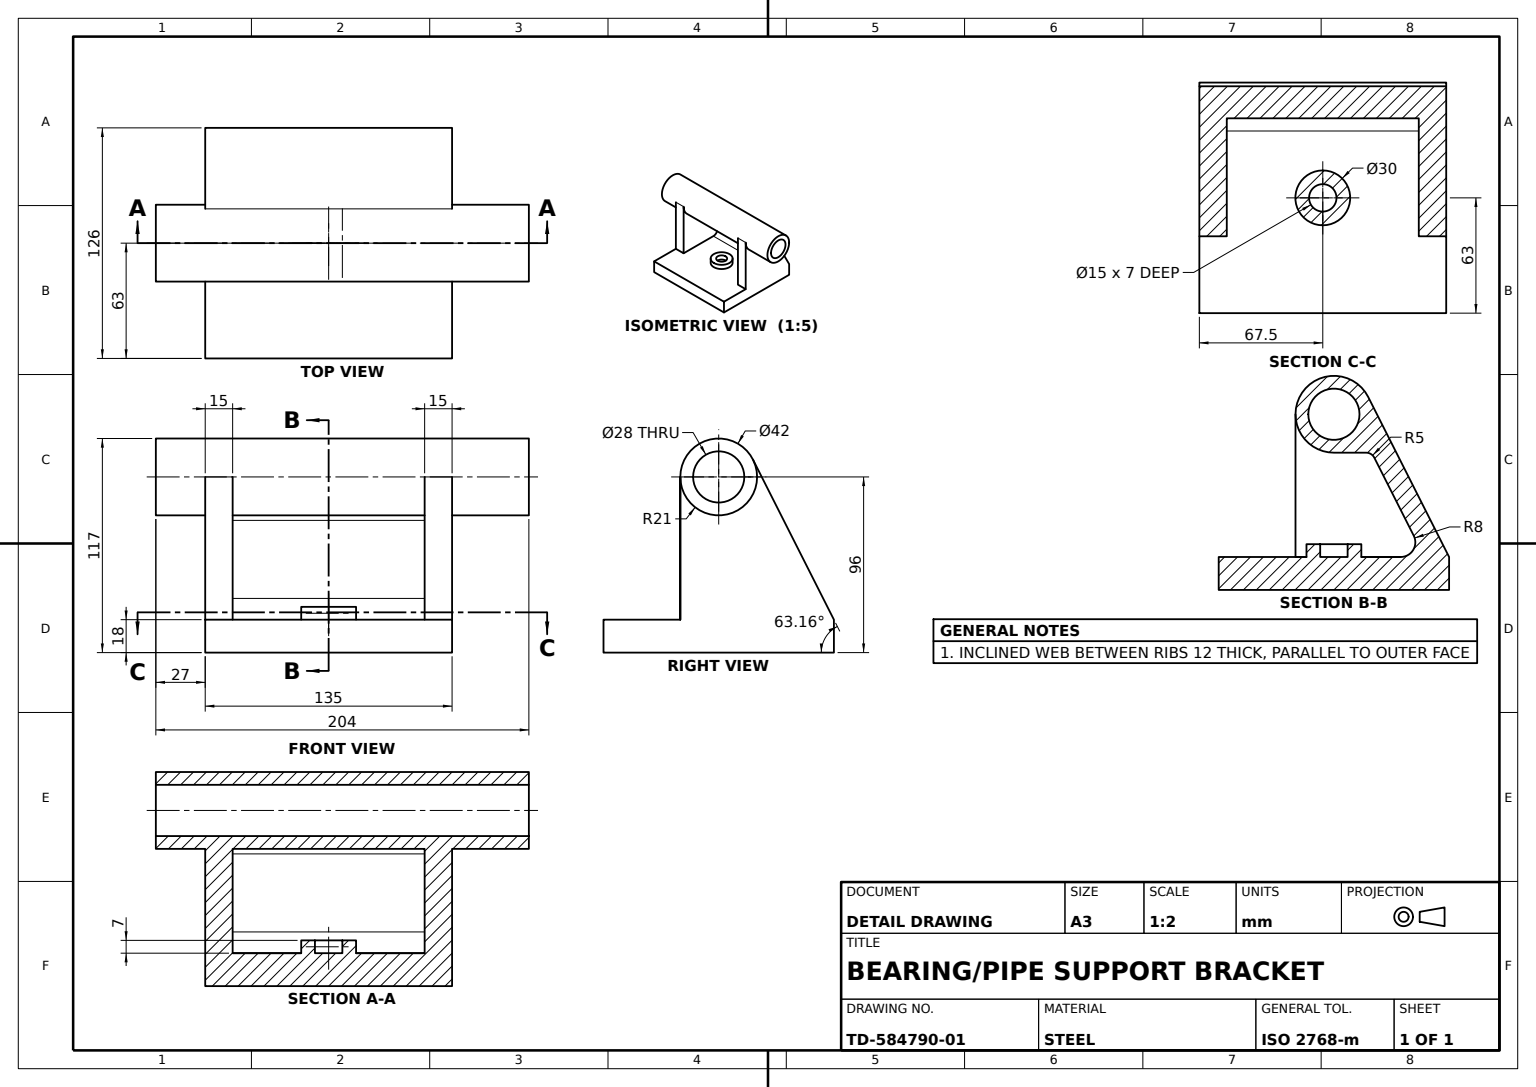
from build123d import *

# Parameters (mm, degrees)
PEDESTAL_SECTION_SKETCH_R              = 14
PEDESTAL_BODY_135MM_DEPTH              = 67.5
TUBE_EXTENSION_SHORT_SKETCH_42X_28_R   = 21
TUBE_EXTENSION_SHORT_SKETCH_42X_28_R_2 = 14
TUBE_EXTENSION_27MM_DEPTH              = 27
TUBE_START                             = 42
TUBE_EXTENSION_LONG_SKETCH_42X_28_R    = 21
TUBE_EXTENSION_LONG_SKETCH_42X_28_R_2  = 14
TUBE_EXTENSION_42MM_DEPTH              = 42
SUPPORT_RIB_A_DEPTH                    = 15
SUPPORT_START                          = -15
SUPPORT_RIB_B_DEPTH                    = 15
BASE_BOSS_SKETCH_30X_15_R              = 15
BASE_BOSS_SKETCH_30X_15_R_2            = 7.5
BASE_BOSS_30X_15_DEPTH                 = 7


with BuildPart() as part:
    # Pedestal Section Sketch → Pedestal Body 135mm (new, symmetric)
    with BuildSketch(Plane(origin=(0, 0, 0), x_dir=(0, 0, -1), z_dir=(1, 0, 0))):
        with BuildLine():
            Line((-63, 18), (-63, 0))
            Line((-63, 0), (63, 0))
            Line((63, 0), (63, 18))
            Line((63, 18), (18.738072538, 105.480750896))
            ThreePointArc((18.738072538, 105.480750896), (-17.88988218, 106.997823221), (0, 75))
            Line((0, 75), (17.637861238, 75))
            ThreePointArc((17.637861238, 75), (20.256390577, 74.259495757), (22.099307081, 72.257321642))
            Line((22.099307081, 72.257321642), (43.676359689, 29.611714627))
            ThreePointArc((43.676359689, 29.611714627), (43.353239552, 21.810353059), (36.538046341, 18))
            Line((36.538046341, 18), (-63, 18))
        make_face()
        with Locations((0, 96)):
            Circle(PEDESTAL_SECTION_SKETCH_R, mode=Mode.SUBTRACT)
    extrude(amount=PEDESTAL_BODY_135MM_DEPTH, both=True)

    # Tube Extension Short Sketch Ø42xØ28 → Tube Extension 27mm (add)
    with BuildSketch(Plane.ZY.offset(67.5)):
        with Locations((0, 96)):
            Circle(TUBE_EXTENSION_SHORT_SKETCH_42X_28_R)
        with Locations((0, 96)):
            Circle(TUBE_EXTENSION_SHORT_SKETCH_42X_28_R_2, mode=Mode.SUBTRACT)
    extrude(amount=TUBE_EXTENSION_27MM_DEPTH)

    # Tube Extension Long Sketch Ø42xØ28 → Tube Extension 42mm (add)
    with BuildSketch(Plane(origin=(67.5, 0, 0), x_dir=(0, 0, -1), z_dir=(1, 0, 0)).offset(TUBE_START)):
        with Locations(Location((0, 96, 0), (0, 0, 180))):
            Circle(TUBE_EXTENSION_LONG_SKETCH_42X_28_R)
        with Locations(Location((0, 96, 0), (0, 0, 180))):
            Circle(TUBE_EXTENSION_LONG_SKETCH_42X_28_R_2, mode=Mode.SUBTRACT)
    extrude(amount=-TUBE_EXTENSION_42MM_DEPTH)

    # Support Rib A Sketch → Support Rib A (add)
    with BuildSketch(Plane(origin=(67.5, 0, 0), x_dir=(0, 0, -1), z_dir=(1, 0, 0))):
        with BuildLine():
            Line((-21, 96), (-21, 18))
            Line((-21, 18), (36.538046341, 18))
            ThreePointArc((36.538046341, 18), (43.353239552, 21.810353059), (43.676359689, 29.611714627))
            Line((43.676359689, 29.611714627), (22.099307081, 72.257321642))
            ThreePointArc((22.099307081, 72.257321642), (20.256390577, 74.259495757), (17.637861238, 75))
            Line((17.637861238, 75), (0, 75))
            ThreePointArc((0, 75), (-14.849242405, 81.150757595), (-21, 96))
        make_face()
    extrude(amount=-SUPPORT_RIB_A_DEPTH)

    # Support Rib B Sketch → Support Rib B (add)
    with BuildSketch(Plane.ZY.offset(67.5).offset(SUPPORT_START)):
        with BuildLine():
            Line((21, 96), (21, 18))
            Line((21, 18), (-36.538046341, 18))
            ThreePointArc((-36.538046341, 18), (-43.353239552, 21.810353059), (-43.676359689, 29.611714627))
            Line((-43.676359689, 29.611714627), (-22.099307081, 72.257321642))
            ThreePointArc((-22.099307081, 72.257321642), (-20.256390577, 74.259495757), (-17.637861238, 75))
            Line((-17.637861238, 75), (0, 75))
            ThreePointArc((0, 75), (14.849242405, 81.150757595), (21, 96))
        make_face()
    extrude(amount=SUPPORT_RIB_B_DEPTH)

    # Base Boss Sketch Ø30xØ15 → Base Boss Ø30xØ15 (add)
    with BuildSketch(Plane(origin=(0, 18, 0), x_dir=(1, 0, 0), z_dir=(0, 1, 0))):
        with Locations(Location((0, 0, 0), (0, 0, 270))):
            Circle(BASE_BOSS_SKETCH_30X_15_R)
        with Locations(Location((0, 0, 0), (0, 0, 270))):
            Circle(BASE_BOSS_SKETCH_30X_15_R_2, mode=Mode.SUBTRACT)
    extrude(amount=BASE_BOSS_30X_15_DEPTH)


solid = part.part
